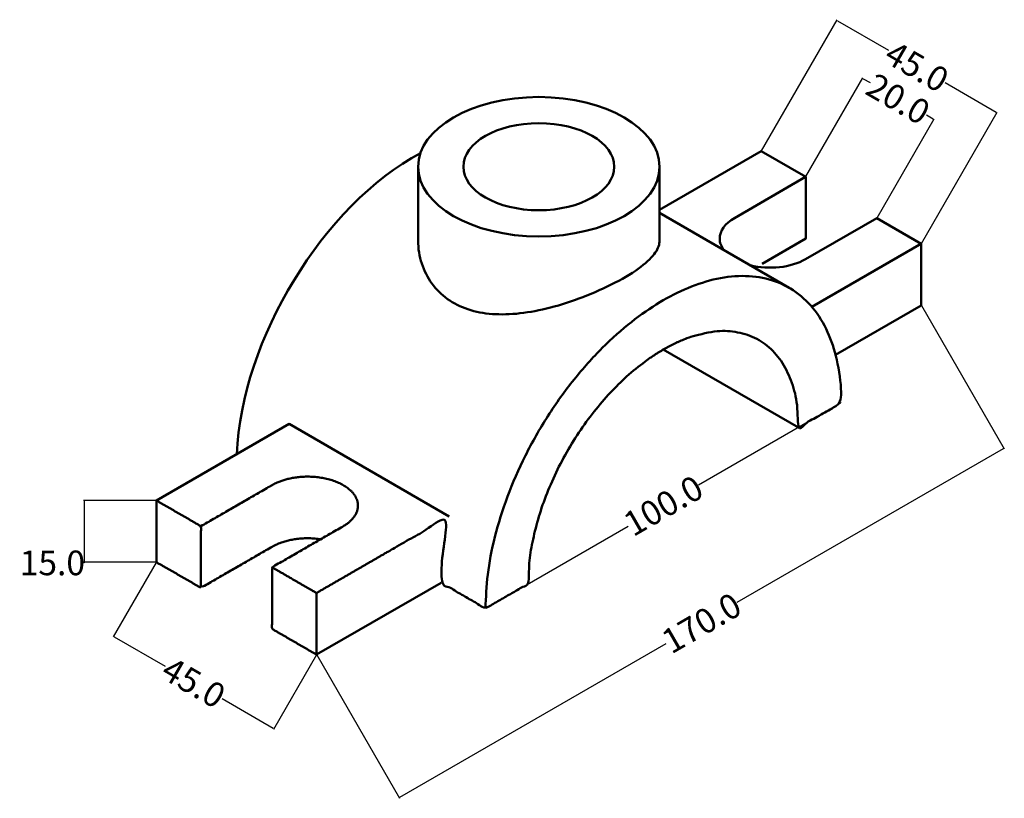
# Model space of a CAD drawing. Units: millimetres. Extents: x -20 to 220, y -2 to 187.
import ezdxf

# ---------------------------------------------------------------- set-up
doc = ezdxf.new("R2010")
doc.units = ezdxf.units.MM
doc.header["$MEASUREMENT"] = 0
doc.layers.add('M-DIMS', color=2, linetype='Continuous', lineweight=25)
doc.layers.add('M-OUTL', color=7, linetype='Continuous', lineweight=50)
doc.styles.get("Standard").update_dxf_attribs({"font": 'arial.ttf'})
doc.dimstyles.get("Standard").update_dxf_attribs({"dimtxt": 6, "dimasz": 0.18, "dimexe": 0.18, "dimexo": 0.0625, "dimgap": 0.09, "dimtad": 0, "dimtoh": 1, "dimdec": 1, "dimzin": 0, "dimdsep": 46, "dimtxsty": 'Standard', "dimcen": 0.09, "dimadec": 0, "dimazin": 0, "dimtfac": 1, "dimtdec": 1, "dimtofl": 0, "dimtmove": 0, "dimatfit": 3, "dimfxl": 1, "dimtolj": 1, "dimtzin": 0, "dimarcsym": 0})

# ---------------------------------------------------------------- blocks, each defined once
blk = doc.blocks.new('*D1')
at = {"layer": 'Defpoints', "color": 0, "transparency": 16777216}
for p in [(199.99, 117.57), (220.1, 82.75), (52.73, 32.55)]:
    blk.add_point(p, dxfattribs=at)
at = {"layer": 'M-DIMS', "color": 0, "lineweight": -2, "transparency": 16777216}
for p, q in [((200.03, 117.52), (220.19, 82.6)), ((219.94, 82.66), (155.06, 45.2)), ((72.99, -2.18), (137.88, 35.28)), ((52.77, 32.5), (72.93, -2.42))]:
    blk.add_line(p, q, dxfattribs=at)
at = {"layer": 'M-DIMS', "color": 0, "transparency": 16777216}
for points in [[(219.93, 82.69), (219.96, 82.64), (220.1, 82.75)], [(72.98, -2.15), (73.01, -2.2), (72.84, -2.27)]]:
    blk.add_solid(points, dxfattribs=at)
at = {"layer": 'M-DIMS', "color": 0, "transparency": 16777216, "insert": (146.47, 40.24), "char_height": 6, "attachment_point": 5, "rotation": 30}
blk.add_mtext('\\A1;170.0', dxfattribs=at)
blk = doc.blocks.new('*D2')
at = {"layer": 'Defpoints', "color": 0, "transparency": 16777216}
for p in [(13.76, 55.05), (52.73, 32.55), (42.31, 14.49)]:
    blk.add_point(p, dxfattribs=at)
at = {"layer": 'M-DIMS', "color": 0, "lineweight": -2, "transparency": 16777216}
for p, q in [((13.73, 55), (3.25, 36.84)), ((3.49, 36.9), (15.9, 29.74)), ((52.7, 32.5), (42.22, 14.34)), ((42.15, 14.58), (29.75, 21.75))]:
    blk.add_line(p, q, dxfattribs=at)
at = {"layer": 'M-DIMS', "color": 0, "transparency": 16777216}
for points in [[(3.51, 36.93), (3.48, 36.88), (3.34, 36.99)], [(42.17, 14.61), (42.14, 14.56), (42.31, 14.49)]]:
    blk.add_solid(points, dxfattribs=at)
at = {"layer": 'M-DIMS', "color": 0, "transparency": 16777216, "insert": (22.82, 25.74), "char_height": 6, "attachment_point": 5, "rotation": 330}
blk.add_mtext('\\A1;45.0', dxfattribs=at)
blk = doc.blocks.new('*D3')
at = {"layer": 'Defpoints', "color": 0, "transparency": 16777216}
for p in [(203.01, 162.8), (171.85, 148.82), (189.17, 138.82)]:
    blk.add_point(p, dxfattribs=at)
at = {"layer": 'M-DIMS', "color": 0, "lineweight": -2, "transparency": 16777216}
for p, q in [((171.88, 148.88), (185.78, 172.95)), ((185.85, 172.71), (187.49, 171.76)), ((202.85, 162.89), (201.21, 163.83)), ((189.2, 138.88), (203.1, 162.95))]:
    blk.add_line(p, q, dxfattribs=at)
at = {"layer": 'M-DIMS', "color": 0, "transparency": 16777216}
for points in [[(185.86, 172.73), (185.83, 172.68), (185.69, 172.8)], [(202.87, 162.91), (202.84, 162.86), (203.01, 162.8)]]:
    blk.add_solid(points, dxfattribs=at)
at = {"layer": 'M-DIMS', "color": 0, "transparency": 16777216, "insert": (194.35, 167.8), "char_height": 6, "attachment_point": 5, "rotation": 330}
blk.add_mtext('\\A1;20.0', dxfattribs=at)
blk = doc.blocks.new('*D4')
at = {"layer": 'Defpoints', "color": 0, "transparency": 16777216}
for p in [(218.38, 164.42), (161.02, 155.07), (199.99, 132.57)]:
    blk.add_point(p, dxfattribs=at)
at = {"layer": 'M-DIMS', "color": 0, "lineweight": -2, "transparency": 16777216}
for p, q in [((161.05, 155.13), (179.5, 187.08)), ((179.57, 186.83), (191.98, 179.67)), ((218.23, 164.51), (205.82, 171.68)), ((200.03, 132.63), (218.47, 164.58))]:
    blk.add_line(p, q, dxfattribs=at)
at = {"layer": 'M-DIMS', "color": 0, "transparency": 16777216}
for points in [[(179.58, 186.86), (179.55, 186.81), (179.41, 186.92)], [(218.24, 164.54), (218.21, 164.49), (218.38, 164.42)]]:
    blk.add_solid(points, dxfattribs=at)
at = {"layer": 'M-DIMS', "color": 0, "transparency": 16777216, "insert": (198.9, 175.67), "char_height": 6, "attachment_point": 5, "rotation": 330}
blk.add_mtext('\\A1;45.0', dxfattribs=at)
blk = doc.blocks.new('*D5')
at = {"layer": 'Defpoints', "color": 0, "transparency": 16777216}
for p in [(13.76, 70.05), (-3.81, 55.05), (13.76, 55.05)]:
    blk.add_point(p, dxfattribs=at)
at = {"layer": 'M-DIMS', "color": 0, "lineweight": -2, "transparency": 16777216}
for p, q in [((13.7, 70.05), (-3.99, 70.05)), ((-3.81, 69.87), (-3.81, 55.23)), ((13.7, 55.05), (-3.99, 55.05)), ((-3.81, 54.87), (-3.99, 54.87)), ((-3.81, 55.05), (-3.81, 54.87))]:
    blk.add_line(p, q, dxfattribs=at)
at = {"layer": 'M-DIMS', "color": 0, "transparency": 16777216}
for points in [[(-3.84, 69.87), (-3.78, 69.87), (-3.81, 70.05)], [(-3.84, 55.23), (-3.78, 55.23), (-3.81, 55.05)]]:
    blk.add_solid(points, dxfattribs=at)
at = {"layer": 'M-DIMS', "color": 0, "transparency": 16777216, "insert": (-11.58, 54.87), "char_height": 6, "attachment_point": 5}
blk.add_mtext('\\A1;15.0', dxfattribs=at)
blk = doc.blocks.new('*D6')
at = {"layer": 'Defpoints', "color": 0, "transparency": 16777216}
for p in [(180.47, 93.8), (180.47, 93.8), (93.87, 43.8)]:
    blk.add_point(p, dxfattribs=at)
at = {"layer": 'M-DIMS', "color": 0, "lineweight": -2, "transparency": 16777216}
for p, q in [((180.32, 93.71), (145.76, 73.76)), ((180.44, 93.86), (180.38, 93.96)), ((94.03, 43.89), (128.58, 63.84)), ((93.84, 43.86), (93.78, 43.96))]:
    blk.add_line(p, q, dxfattribs=at)
at = {"layer": 'M-DIMS', "color": 0, "transparency": 16777216}
for points in [[(180.3, 93.74), (180.33, 93.69), (180.47, 93.8)], [(94.01, 43.92), (94.04, 43.87), (93.87, 43.8)]]:
    blk.add_solid(points, dxfattribs=at)
at = {"layer": 'M-DIMS', "color": 0, "transparency": 16777216, "insert": (137.17, 68.8), "char_height": 6, "attachment_point": 5, "rotation": 30}
blk.add_mtext('\\A1;100.0', dxfattribs=at)

msp = doc.modelspace()

# ---------------------------------------------------------------- linework, layer by layer
at = {"layer": 'M-OUTL'}
for p, q in [((77.47, 133.33), (77.47, 151.3)), ((136.26, 133.33), (136.26, 151.3)), ((154.49, 138.8), (171.81, 148.8)), ((167.79, 121.84), (136.26, 140.04)), ((189.13, 138.8), (171.81, 128.8)), ((199.96, 132.55), (189.13, 138.8)), ((199.99, 132.57), (173.34, 117.18)), ((199.96, 117.55), (199.96, 132.55)), ((179.1, 105.51), (199.96, 117.55)), ((170.08, 87.8), (137.17, 106.8)), ((167.41, 101.26), (167.48, 101.3))]:
    msp.add_line(p, q, dxfattribs=at)
for points in [[(136.26, 140.77), (161.02, 155.07), (171.85, 148.82), (171.85, 133.82), (161.23, 127.69)], [(77.47, 133.33), (77.48, 132.6), (77.53, 131.88), (77.6, 131.16), (77.7, 130.45), (77.82, 129.76), (77.98, 129.07), (78.15, 128.39), (78.36, 127.72), (78.58, 127.07), (78.83, 126.43), (79.11, 125.8), (79.4, 125.19), (79.72, 124.59), (80.07, 124), (80.43, 123.44), (80.82, 122.88), (81.22, 122.35), (81.65, 121.83), (82.1, 121.33), (82.57, 120.84), (83.05, 120.38), (83.56, 119.93), (84.09, 119.51), (84.63, 119.1), (85.19, 118.71), (85.77, 118.35), (86.37, 118), (86.99, 117.68), (87.62, 117.37), (88.26, 117.09), (88.93, 116.83), (89.6, 116.59), (90.3, 116.37), (91.01, 116.18), (91.73, 116), (92.47, 115.85), (93.22, 115.71), (93.98, 115.6), (94.76, 115.51), (95.54, 115.44), (96.34, 115.39), (97.16, 115.37), (97.98, 115.36), (98.82, 115.37), (99.66, 115.4), (100.52, 115.46), (101.39, 115.53), (102.27, 115.62), (103.16, 115.73), (104.06, 115.86), (104.97, 116), (105.89, 116.17), (106.82, 116.36), (107.76, 116.56), (108.71, 116.78), (109.67, 117.02), (110.63, 117.28), (111.61, 117.55), (112.59, 117.84), (113.58, 118.15), (114.57, 118.48), (115.57, 118.83), (116.57, 119.19), (117.57, 119.56), (118.58, 119.96), (119.58, 120.37), (120.58, 120.79), (121.57, 121.22), (122.56, 121.67), (123.53, 122.13), (124.48, 122.6), (125.41, 123.08), (126.32, 123.56), (127.2, 124.05), (128.04, 124.53), (128.86, 125.02), (129.63, 125.51), (130.36, 125.99), (131.04, 126.47), (131.69, 126.94), (132.28, 127.4), (132.83, 127.86), (133.34, 128.3), (133.8, 128.74), (134.22, 129.17), (134.59, 129.58), (134.92, 129.99), (135.22, 130.39), (135.47, 130.78), (135.68, 131.17), (135.86, 131.54), (136.01, 131.91), (136.12, 132.28), (136.19, 132.63), (136.24, 132.99), (136.26, 133.33)], [(85.04, 66.2), (46.07, 88.7), (13.76, 70.05)], [(52.73, 47.55), (52.73, 32.55), (83.05, 50.05)]]:
    msp.add_lwpolyline(points, dxfattribs=at)
for major_axis in [(-29.39, 0), (-18.37, 0)]:
    msp.add_ellipse((106.86, 151.3), major_axis=major_axis, ratio=0.57735, dxfattribs=at)
for centre, major_axis, start_param, end_param in [((76.55, 103.8), (-30.62, -53.03), 3.892612, 5.447766), ((163.15, 133.8), (-12.25, 0), 5.497787, 6.283185), ((163.15, 133.8), (-12.25, 0), 0, 0.40612), ((163.15, 133.8), (-12.25, 0), 1.164676, 2.356194)]:
    msp.add_ellipse(centre, major_axis=major_axis, ratio=0.57735, start_param=start_param, end_param=end_param, dxfattribs=at)
for points, weights, knots in [([(44.07, 52.55), (42.99, 53.18), (41.91, 53.8), (47.32, 50.68), (52.73, 47.55), (68.89, 56.88), (85.04, 66.2), (83.05, 57.73), (83.05, 50.05), (88.46, 46.93), (93.87, 43.8), (99.07, 46.8), (104.26, 49.8), (104.26, 87.8), (137.17, 106.8), (170.08, 125.8), (170.08, 87.8), (175.28, 90.8), (180.47, 93.8), (180.47, 143.8), (137.17, 118.8), (93.87, 93.8), (93.87, 43.8)], [1, 1, 1, 1, 1, 1, 1, 0.988417725817, 1, 1, 1, 1, 1, 0.707106781187, 1, 0.707106781187, 1, 1, 1, 0.707106781187, 1, 0.707106781187, 1], [0, 0, 0, 1, 1, 2, 2, 3, 3, 3.304693, 3.304693, 4.304693, 4.304693, 5.304693, 5.304693, 6.875489, 6.875489, 8.446285, 8.446285, 9.446285, 9.446285, 11.017082, 11.017082, 12.587878, 12.587878, 12.587878]), ([(52.73, 32.55), (47.32, 35.68), (41.91, 38.8), (41.91, 46.3), (41.91, 53.8), (50.57, 58.8), (59.23, 63.8), (64.23, 66.69), (62.4, 70.63), (60.57, 74.58), (53.74, 75.63), (46.91, 76.69), (41.91, 73.8), (33.25, 68.8), (24.59, 63.8)], [1, 1, 1, 1, 1, 1, 1, 0.866025403784, 1, 0.866025403784, 1, 0.866025403784, 1, 1, 1], [0, 0, 0, 1, 1, 2, 2, 3, 3, 4.047198, 4.047198, 5.094395, 5.094395, 6.141593, 6.141593, 7.141593, 7.141593, 7.141593]), ([(53.74, 60.63), (46.91, 61.69), (41.91, 58.8), (33.25, 53.8), (24.59, 48.8), (24.59, 56.3), (24.59, 63.8), (19.18, 66.93), (13.76, 70.05), (13.76, 62.55), (13.76, 55.05), (19.18, 51.93), (24.59, 48.8)], [1, 0.866025403784, 1, 1, 1, 1, 1, 1, 1, 1, 1, 1, 1], [0, 0, 0, 1.047198, 1.047198, 2.047198, 2.047198, 3.047198, 3.047198, 4.047198, 4.047198, 5.047198, 5.047198, 6.047198, 6.047198, 6.047198])]:
    msp.add_rational_spline(points, weights, degree=2, knots=knots, dxfattribs=at)

# ---------------------------------------------------------------- dimensions: what is measured, and where the dimension line sits
at = {"layer": 'M-DIMS'}
for p1, p2, distance, picture, middle in [((161.02, 155.07), (199.99, 132.57), 36.78, '*D4', (198.9, 175.67)), ((171.85, 148.82), (189.17, 138.82), 27.68, '*D3', (194.35, 167.8)), ((52.73, 32.55), (199.99, 117.57), -40.21, '*D1', (146.47, 40.24)), ((93.87, 43.8), (180.47, 93.8), 0, '*D6', (137.17, 68.8)), ((13.76, 70.05), (13.76, 55.05), -17.58, '*D5', (-11.58, 54.87)), ((13.76, 55.05), (52.73, 32.55), -20.85, '*D2', (22.82, 25.74))]:
    dim = msp.add_aligned_dim(p1=p1, p2=p2, distance=distance, dimstyle='Standard', override={"dimclrd": 0, "dimclre": 0, "dimclrt": 0}, dxfattribs=at)
    dim.commit()
    dim.dimension.update_dxf_attribs({"geometry": picture, "text_midpoint": middle})

doc.saveas('drawing.dxf')
